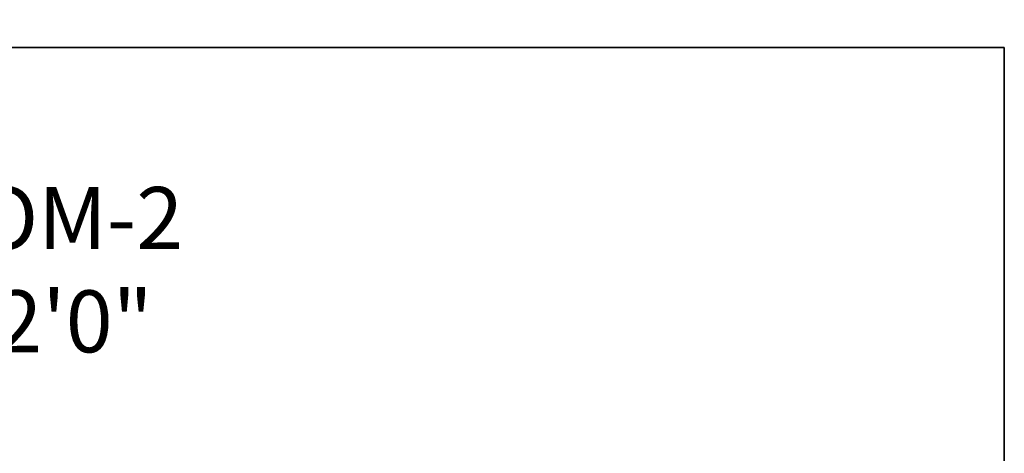
# Model space of a CAD drawing. Units: inches. Extents: x 1484 to 2008, y 1843 to 2590.
# Tile 9 of 21: x 1811 to 1891, y 2040 to 2075. Entities that reach past the tile are written whole.
import ezdxf

# ---------------------------------------------------------------- set-up
doc = ezdxf.new("R2010")
doc.units = ezdxf.units.IN
for name, color, linetype, lineweight in [('A-ANNO-DIMS', 2, 'Continuous', 18), ('A-AREA-IDEN', 7, 'Continuous', 18), ('A-WALL', 7, 'Continuous', 35)]:
    doc.layers.add(name, color=color, linetype=linetype, lineweight=lineweight)
doc.styles.get("Standard").update_dxf_attribs({"font": 'arial.ttf'})
doc.dimstyles.new('ISO-25', dxfattribs={"dimtxt": 7, "dimasz": 2.5, "dimexe": 1.25, "dimexo": 0.625, "dimtad": 1, "dimdec": 0, "dimlunit": 3, "dimtxsty": 'Standard', "dimcen": 2.5, "dimadec": 0, "dimazin": 0, "dimtfac": 1, "dimtdec": 0, "dimtmove": 0, "dimatfit": 3, "dimfxl": 1, "dimarcsym": 0})

# ---------------------------------------------------------------- blocks, each defined once
blk = doc.blocks.new('*D11')
at = {"layer": 'A-ANNO-DIMS', "color": 0, "lineweight": -2, "transparency": 16777216}
for p, q in [((1754.42, 2083.338), (1754.42, 2076.976)), ((1792.67, 2083.338), (1792.67, 2076.976)), ((1756.92, 2078.226), (1790.17, 2078.226)), ((1792.67, 2078.226), (1887.105, 2078.226))]:
    blk.add_line(p, q, dxfattribs=at)
at = {"layer": 'A-ANNO-DIMS', "color": 0, "transparency": 16777216}
for points in [[(1756.92, 2078.642), (1756.92, 2077.809), (1754.42, 2078.226)], [(1790.17, 2078.642), (1790.17, 2077.809), (1792.67, 2078.226)]]:
    blk.add_solid(points, dxfattribs=at)
at = {"layer": 'Defpoints', "color": 0, "transparency": 16777216}
for p in [(1754.42, 2083.963), (1792.67, 2083.963), (1792.67, 2078.226)]:
    blk.add_point(p, dxfattribs=at)
at = {"layer": 'A-ANNO-DIMS', "color": 0, "transparency": 16777216, "insert": (1841.137, 2082.475), "char_height": 7, "attachment_point": 5}
blk.add_mtext('DOOR 3\'-2 1/2" TYP.', dxfattribs=at)

msp = doc.modelspace()

# ---------------------------------------------------------------- linework, layer by layer
at = {"layer": 'A-WALL'}
for p, q in [((1758.92, 2072.803), (1890.92, 2072.803)), ((1890.92, 2072.803), (1890.92, 1928.803))]:
    msp.add_line(p, q, dxfattribs=at)

# ---------------------------------------------------------------- texts
at = {"layer": 'A-AREA-IDEN', "insert": (1785.341, 2061.564), "char_height": 5, "attachment_point": 1}
msp.add_mtext_dynamic_manual_height_columns('BEDROOM-2\\P11\'0"X12\'0"', width=40.96888, gutter_width=12.5, heights=[0], dxfattribs=at)

# ---------------------------------------------------------------- dimensions: what is measured, and where the dimension line sits
at = {"layer": 'A-ANNO-DIMS'}
dim = msp.add_linear_dim(base=(1792.669643705, 2078.225576395), p1=(1754.419643705, 2083.963076395), p2=(1792.669643705, 2083.963076395), text='DOOR <> TYP.', dimstyle='ISO-25', override={"dimdec": 1, "dimlfac": 1, "dimrnd": 0, "dimzin": 1, "dimdsep": 46, "dimlunit": 4, "dimfrac": 2}, dxfattribs=at)
dim.commit()
dim.dimension.update_dxf_attribs({"geometry": '*D11', "text_midpoint": (1841.137072082, 2082.474723734)})

doc.saveas('drawing.dxf')
